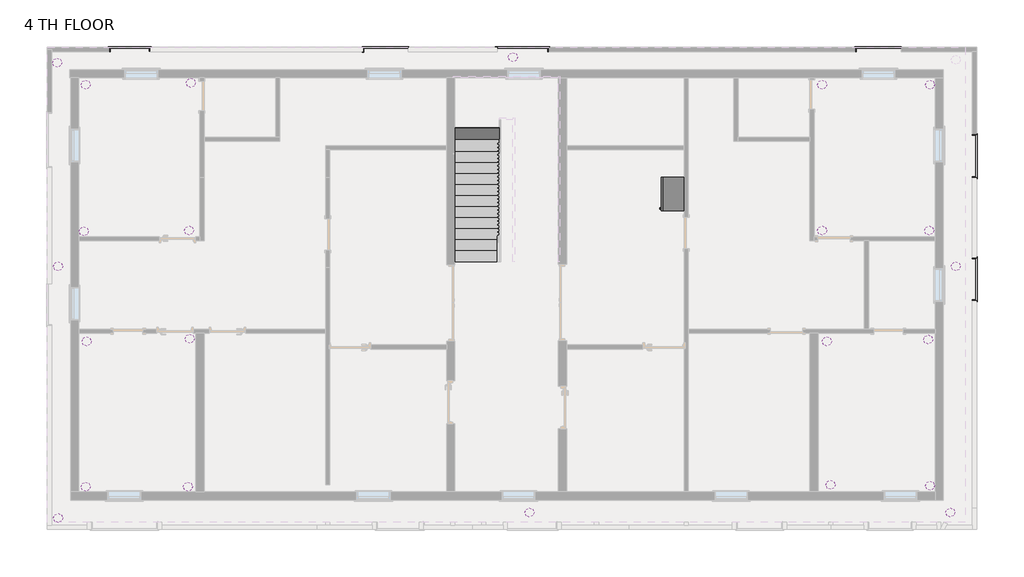
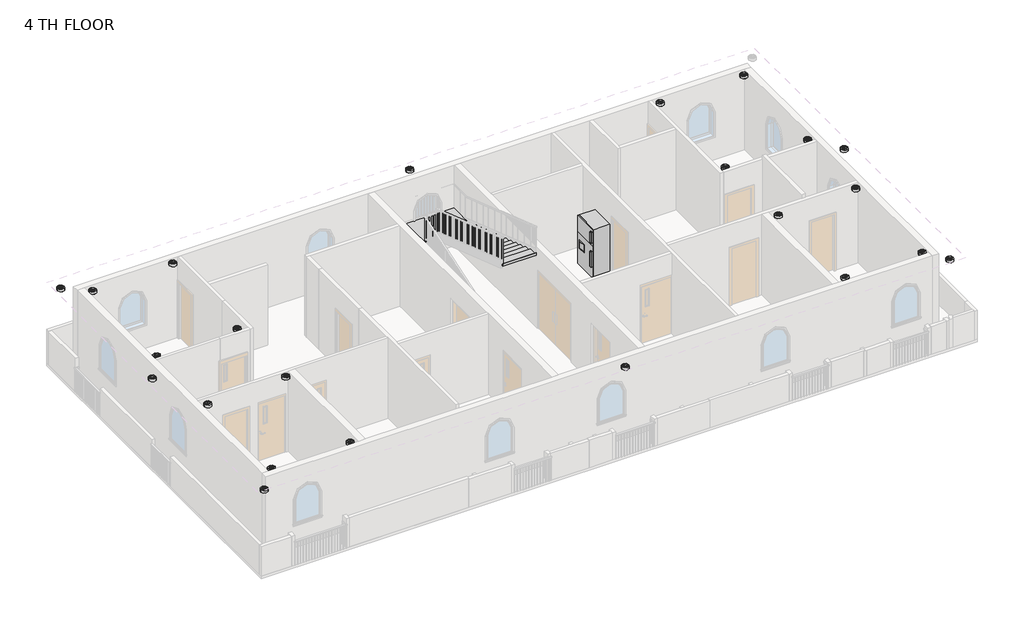
# One storey, part 6 of 7: 23 light fixtures, 6 railings, 1 furniture element, 1 stair flight.
"""IFC4 building model written with IfcOpenShell, lengths in millimetres."""

from ifc_helpers import new_model, si_unit, frame, origin, place, context, project, spatial, polyline, outline, extrude, faceted_brep, transform, mapped, element, save
from components import furniture_65fa61b5, ceiling_light_flat_round_60w_120v_7c4c2a52, stair_flight_ccf7fef2

model = new_model("IFC4")

# Units and contexts
model_context = context("Model", 3, world=origin())
ifc_project = project(units=[si_unit("LENGTHUNIT", "METRE", prefix="MILLI")], contexts=[model_context])

# Site, building, storey
site = spatial("IfcSite", under=ifc_project)
building = spatial("IfcBuilding", under=site)
storey = spatial("IfcBuildingStorey", under=building, Name="4 TH FLOOR", Elevation=12801.6)

# Furniture
placement = place(None, origin())
furniture_shape = furniture_65fa61b5(model_context)
element("IfcFurniture", 1, at=placement, inside=storey, context=model_context, shape_type="MappedRepresentation", body=[
    mapped(furniture_shape, transform((4507.551208, 3815.4567334, 12801.6), x_axis=(0.0, -1.0, 0.0), y_axis=(1.0, 0.0, 0.0), z_axis=(0.0, 0.0, 1.0))),
])

# Light fixtures
ceiling_light_flat_round_60w_120v_shape = ceiling_light_flat_round_60w_120v_7c4c2a52(model_context)
element("IfcLightFixture", 2, ObjectType="Ceiling Light - Flat Round : 60W - 120V", at=placement, inside=storey, context=model_context, shape_type="MappedRepresentation", body=[
    mapped(ceiling_light_flat_round_60w_120v_shape, transform((-12821.5987925, 8050.9067329, 13411.2), x_axis=(1.0, 0.0, 0.0), y_axis=(0.0, 1.0, 0.0), z_axis=(0.0, 0.0, 1.0))),
])
element("IfcLightFixture", 3, ObjectType="Ceiling Light - Flat Round : 60W - 120V", at=placement, inside=storey, context=model_context, shape_type="MappedRepresentation", body=[
    mapped(ceiling_light_flat_round_60w_120v_shape, transform((-249.1067989, 8203.3067329, 13411.2), x_axis=(1.0, 0.0, 0.0), y_axis=(0.0, 1.0, 0.0), z_axis=(0.0, 0.0, 1.0))),
])
element("IfcLightFixture", 4, ObjectType="Ceiling Light - Flat Round : 60W - 120V", at=placement, inside=storey, context=model_context, shape_type="MappedRepresentation", body=[
    mapped(ceiling_light_flat_round_60w_120v_shape, transform((-12796.1987925, -4509.3932193, 13411.2), x_axis=(1.0, 0.0, 0.0), y_axis=(0.0, 1.0, 0.0), z_axis=(0.0, 0.0, 1.0))),
])
element("IfcLightFixture", 5, ObjectType="Ceiling Light - Flat Round : 60W - 120V", at=placement, inside=storey, context=model_context, shape_type="MappedRepresentation", body=[
    mapped(ceiling_light_flat_round_60w_120v_shape, transform((-12796.1987925, 2431.1567332, 13411.2), x_axis=(1.0, 0.0, 0.0), y_axis=(0.0, 1.0, 0.0), z_axis=(0.0, 0.0, 1.0))),
])
element("IfcLightFixture", 6, ObjectType="Ceiling Light - Flat Round : 60W - 120V", at=placement, inside=storey, context=model_context, shape_type="MappedRepresentation", body=[
    mapped(ceiling_light_flat_round_60w_120v_shape, transform((208.0932011, -4356.9932193, 13411.2), x_axis=(1.0, 0.0, 0.0), y_axis=(0.0, 1.0, 0.0), z_axis=(0.0, 0.0, 1.0))),
])
element("IfcLightFixture", 7, ObjectType="Ceiling Light - Flat Round : 60W - 120V", at=placement, inside=storey, context=model_context, shape_type="MappedRepresentation", body=[
    mapped(ceiling_light_flat_round_60w_120v_shape, transform((11816.4012075, -4356.9932193, 13411.2), x_axis=(1.0, 0.0, 0.0), y_axis=(0.0, 1.0, 0.0), z_axis=(0.0, 0.0, 1.0))),
])
element("IfcLightFixture", 8, ObjectType="Ceiling Light - Flat Round : 60W - 120V", at=placement, inside=storey, context=model_context, shape_type="MappedRepresentation", body=[
    mapped(ceiling_light_flat_round_60w_120v_shape, transform((11968.8012075, 2431.1567332, 13411.2), x_axis=(1.0, 0.0, 0.0), y_axis=(0.0, 1.0, 0.0), z_axis=(0.0, 0.0, 1.0))),
])
element("IfcLightFixture", 9, ObjectType="Ceiling Light - Flat Round : 60W - 120V", at=placement, inside=storey, context=model_context, shape_type="MappedRepresentation", body=[
    mapped(ceiling_light_flat_round_60w_120v_shape, transform((8279.4512079, 7441.3067329, 13411.2), x_axis=(1.0, 0.0, 0.0), y_axis=(0.0, 1.0, 0.0), z_axis=(0.0, 0.0, 1.0))),
])
element("IfcLightFixture", 10, ObjectType="Ceiling Light - Flat Round : 60W - 120V", at=placement, inside=storey, context=model_context, shape_type="MappedRepresentation", body=[
    mapped(ceiling_light_flat_round_60w_120v_shape, transform((11257.6012075, 7441.3067329, 13411.2), x_axis=(1.0, 0.0, 0.0), y_axis=(0.0, 1.0, 0.0), z_axis=(0.0, 0.0, 1.0))),
])
element("IfcLightFixture", 11, ObjectType="Ceiling Light - Flat Round : 60W - 120V", at=placement, inside=storey, context=model_context, shape_type="MappedRepresentation", body=[
    mapped(ceiling_light_flat_round_60w_120v_shape, transform((8279.4512079, 3421.7567332, 13411.2), x_axis=(1.0, 0.0, 0.0), y_axis=(0.0, 1.0, 0.0), z_axis=(0.0, 0.0, 1.0))),
])
element("IfcLightFixture", 12, ObjectType="Ceiling Light - Flat Round : 60W - 120V", at=placement, inside=storey, context=model_context, shape_type="MappedRepresentation", body=[
    mapped(ceiling_light_flat_round_60w_120v_shape, transform((11232.2012075, 3421.7567332, 13411.2), x_axis=(1.0, 0.0, 0.0), y_axis=(0.0, 1.0, 0.0), z_axis=(0.0, 0.0, 1.0))),
])
element("IfcLightFixture", 13, ObjectType="Ceiling Light - Flat Round : 60W - 120V", at=placement, inside=storey, context=model_context, shape_type="MappedRepresentation", body=[
    mapped(ceiling_light_flat_round_60w_120v_shape, transform((8412.8012079, 361.0567334, 13411.2), x_axis=(1.0, 0.0, 0.0), y_axis=(0.0, 1.0, 0.0), z_axis=(0.0, 0.0, 1.0))),
])
element("IfcLightFixture", 14, ObjectType="Ceiling Light - Flat Round : 60W - 120V", at=placement, inside=storey, context=model_context, shape_type="MappedRepresentation", body=[
    mapped(ceiling_light_flat_round_60w_120v_shape, transform((11206.8012075, 411.8567334, 13411.2), x_axis=(1.0, 0.0, 0.0), y_axis=(0.0, 1.0, 0.0), z_axis=(0.0, 0.0, 1.0))),
])
element("IfcLightFixture", 15, ObjectType="Ceiling Light - Flat Round : 60W - 120V", at=placement, inside=storey, context=model_context, shape_type="MappedRepresentation", body=[
    mapped(ceiling_light_flat_round_60w_120v_shape, transform((8514.4012079, -3594.9932193, 13411.2), x_axis=(1.0, 0.0, 0.0), y_axis=(0.0, 1.0, 0.0), z_axis=(0.0, 0.0, 1.0))),
])
element("IfcLightFixture", 16, ObjectType="Ceiling Light - Flat Round : 60W - 120V", at=placement, inside=storey, context=model_context, shape_type="MappedRepresentation", body=[
    mapped(ceiling_light_flat_round_60w_120v_shape, transform((11257.6012075, -3620.3932193, 13411.2), x_axis=(1.0, 0.0, 0.0), y_axis=(0.0, 1.0, 0.0), z_axis=(0.0, 0.0, 1.0))),
])
element("IfcLightFixture", 17, ObjectType="Ceiling Light - Flat Round : 60W - 120V", at=placement, inside=storey, context=model_context, shape_type="MappedRepresentation", body=[
    mapped(ceiling_light_flat_round_60w_120v_shape, transform((-12008.7987925, 361.0567334, 13411.2), x_axis=(1.0, 0.0, 0.0), y_axis=(0.0, 1.0, 0.0), z_axis=(0.0, 0.0, 1.0))),
])
element("IfcLightFixture", 18, ObjectType="Ceiling Light - Flat Round : 60W - 120V", at=placement, inside=storey, context=model_context, shape_type="MappedRepresentation", body=[
    mapped(ceiling_light_flat_round_60w_120v_shape, transform((-9163.9987992, 437.2567334, 13411.2), x_axis=(1.0, 0.0, 0.0), y_axis=(0.0, 1.0, 0.0), z_axis=(0.0, 0.0, 1.0))),
])
element("IfcLightFixture", 19, ObjectType="Ceiling Light - Flat Round : 60W - 120V", at=placement, inside=storey, context=model_context, shape_type="MappedRepresentation", body=[
    mapped(ceiling_light_flat_round_60w_120v_shape, transform((-12034.1987925, -3645.7932193, 13411.2), x_axis=(1.0, 0.0, 0.0), y_axis=(0.0, 1.0, 0.0), z_axis=(0.0, 0.0, 1.0))),
])
element("IfcLightFixture", 20, ObjectType="Ceiling Light - Flat Round : 60W - 120V", at=placement, inside=storey, context=model_context, shape_type="MappedRepresentation", body=[
    mapped(ceiling_light_flat_round_60w_120v_shape, transform((-9214.7987992, -3645.7932193, 13411.2), x_axis=(1.0, 0.0, 0.0), y_axis=(0.0, 1.0, 0.0), z_axis=(0.0, 0.0, 1.0))),
])
element("IfcLightFixture", 21, ObjectType="Ceiling Light - Flat Round : 60W - 120V", at=placement, inside=storey, context=model_context, shape_type="MappedRepresentation", body=[
    mapped(ceiling_light_flat_round_60w_120v_shape, transform((-12034.1987925, 7441.3067329, 13411.2), x_axis=(1.0, 0.0, 0.0), y_axis=(0.0, 1.0, 0.0), z_axis=(0.0, 0.0, 1.0))),
])
element("IfcLightFixture", 22, ObjectType="Ceiling Light - Flat Round : 60W - 120V", at=placement, inside=storey, context=model_context, shape_type="MappedRepresentation", body=[
    mapped(ceiling_light_flat_round_60w_120v_shape, transform((-9132.2487992, 7492.1067329, 13411.2), x_axis=(1.0, 0.0, 0.0), y_axis=(0.0, 1.0, 0.0), z_axis=(0.0, 0.0, 1.0))),
])
element("IfcLightFixture", 23, ObjectType="Ceiling Light - Flat Round : 60W - 120V", at=placement, inside=storey, context=model_context, shape_type="MappedRepresentation", body=[
    mapped(ceiling_light_flat_round_60w_120v_shape, transform((-12084.9987925, 3396.3567332, 13411.2), x_axis=(1.0, 0.0, 0.0), y_axis=(0.0, 1.0, 0.0), z_axis=(0.0, 0.0, 1.0))),
])
element("IfcLightFixture", 24, ObjectType="Ceiling Light - Flat Round : 60W - 120V", at=placement, inside=storey, context=model_context, shape_type="MappedRepresentation", body=[
    mapped(ceiling_light_flat_round_60w_120v_shape, transform((-9183.0487992, 3421.7567332, 13411.2), x_axis=(1.0, 0.0, 0.0), y_axis=(0.0, 1.0, 0.0), z_axis=(0.0, 0.0, 1.0))),
])

# Railings
element("IfcRailing", 25, ObjectType="Handrail - Rectangular", at=placement, inside=storey, context=model_context, shape_type="SolidModel", body=[
    faceted_brep([(-11412.4067989, 8355.7067329, 13716.0), (-11412.4067989, 8355.7067329, 13665.2), (-11361.6067989, 8355.7067329, 13665.2), (-11361.6067989, 8355.7067329, 13716.0), (-11412.4067989, 8495.4067329, 13716.0), (-11412.4067989, 8495.4067329, 13665.2), (-11361.6067989, 8444.6067329, 13665.2), (-11361.6067989, 8444.6067329, 13716.0), (-10231.3067989, 8495.4067329, 13716.0), (-10231.3067989, 8495.4067329, 13665.2), (-10282.1067989, 8444.6067329, 13665.2), (-10282.1067989, 8444.6067329, 13716.0), (-10231.3067989, 8368.4067329, 13716.0), (-10282.1067989, 8368.4067329, 13716.0), (-10282.1067989, 8368.4067329, 13665.2), (-10231.3067989, 8368.4067329, 13665.2)], [[[0, 1, 2, 3]], [[1, 0, 4, 5]], [[2, 1, 5, 6]], [[3, 2, 6, 7]], [[0, 3, 7, 4]], [[5, 4, 8, 9]], [[6, 5, 9, 10]], [[7, 6, 10, 11]], [[4, 7, 11, 8]], [[12, 13, 14, 15]], [[9, 8, 12, 15]], [[10, 9, 15, 14]], [[11, 10, 14, 13]], [[8, 11, 13, 12]]]),
    extrude(outline(polyline([(-10278.9317989, 8460.4817329), (-10278.9317989, 8479.5317329), (-10259.8817989, 8479.5317329), (-10259.8817989, 8460.4817329), (-10278.9317989, 8460.4817329)])), frame((0.0, 0.0, 12801.6), z_axis=(0.0, 0.0, 1.0), x_axis=(1.0, 0.0, 0.0)), (0.0, 0.0, 1.0), 863.6),
    extrude(outline(polyline([(-10380.5317989, 8460.4817329), (-10380.5317989, 8479.5317329), (-10361.4817989, 8479.5317329), (-10361.4817989, 8460.4817329), (-10380.5317989, 8460.4817329)])), frame((0.0, 0.0, 12801.6), z_axis=(0.0, 0.0, 1.0), x_axis=(1.0, 0.0, 0.0)), (0.0, 0.0, 1.0), 863.6),
    extrude(outline(polyline([(-10482.1317989, 8460.4817329), (-10482.1317989, 8479.5317329), (-10463.0817989, 8479.5317329), (-10463.0817989, 8460.4817329), (-10482.1317989, 8460.4817329)])), frame((0.0, 0.0, 12801.6), z_axis=(0.0, 0.0, 1.0), x_axis=(1.0, 0.0, 0.0)), (0.0, 0.0, 1.0), 863.6),
    extrude(outline(polyline([(-10583.7317989, 8460.4817329), (-10583.7317989, 8479.5317329), (-10564.6817989, 8479.5317329), (-10564.6817989, 8460.4817329), (-10583.7317989, 8460.4817329)])), frame((0.0, 0.0, 12801.6), z_axis=(0.0, 0.0, 1.0), x_axis=(1.0, 0.0, 0.0)), (0.0, 0.0, 1.0), 863.6),
    extrude(outline(polyline([(-10685.3317989, 8460.4817329), (-10685.3317989, 8479.5317329), (-10666.2817989, 8479.5317329), (-10666.2817989, 8460.4817329), (-10685.3317989, 8460.4817329)])), frame((0.0, 0.0, 12801.6), z_axis=(0.0, 0.0, 1.0), x_axis=(1.0, 0.0, 0.0)), (0.0, 0.0, 1.0), 863.6),
    extrude(outline(polyline([(-10786.9317989, 8460.4817329), (-10786.9317989, 8479.5317329), (-10767.8817989, 8479.5317329), (-10767.8817989, 8460.4817329), (-10786.9317989, 8460.4817329)])), frame((0.0, 0.0, 12801.6), z_axis=(0.0, 0.0, 1.0), x_axis=(1.0, 0.0, 0.0)), (0.0, 0.0, 1.0), 863.6),
    extrude(outline(polyline([(-10888.5317989, 8460.4817329), (-10888.5317989, 8479.5317329), (-10869.4817989, 8479.5317329), (-10869.4817989, 8460.4817329), (-10888.5317989, 8460.4817329)])), frame((0.0, 0.0, 12801.6), z_axis=(0.0, 0.0, 1.0), x_axis=(1.0, 0.0, 0.0)), (0.0, 0.0, 1.0), 863.6),
    extrude(outline(polyline([(-10990.1317989, 8460.4817329), (-10990.1317989, 8479.5317329), (-10971.0817989, 8479.5317329), (-10971.0817989, 8460.4817329), (-10990.1317989, 8460.4817329)])), frame((0.0, 0.0, 12801.6), z_axis=(0.0, 0.0, 1.0), x_axis=(1.0, 0.0, 0.0)), (0.0, 0.0, 1.0), 863.6),
    extrude(outline(polyline([(-11091.7317989, 8460.4817329), (-11091.7317989, 8479.5317329), (-11072.6817989, 8479.5317329), (-11072.6817989, 8460.4817329), (-11091.7317989, 8460.4817329)])), frame((0.0, 0.0, 12801.6), z_axis=(0.0, 0.0, 1.0), x_axis=(1.0, 0.0, 0.0)), (0.0, 0.0, 1.0), 863.6),
    extrude(outline(polyline([(-11193.3317989, 8460.4817329), (-11193.3317989, 8479.5317329), (-11174.2817989, 8479.5317329), (-11174.2817989, 8460.4817329), (-11193.3317989, 8460.4817329)])), frame((0.0, 0.0, 12801.6), z_axis=(0.0, 0.0, 1.0), x_axis=(1.0, 0.0, 0.0)), (0.0, 0.0, 1.0), 863.6),
    extrude(outline(polyline([(-11294.9317989, 8460.4817329), (-11294.9317989, 8479.5317329), (-11275.8817989, 8479.5317329), (-11275.8817989, 8460.4817329), (-11294.9317989, 8460.4817329)])), frame((0.0, 0.0, 12801.6), z_axis=(0.0, 0.0, 1.0), x_axis=(1.0, 0.0, 0.0)), (0.0, 0.0, 1.0), 863.6),
    extrude(outline(polyline([(-11377.4817989, 8447.7817329), (-11396.5317989, 8447.7817329), (-11396.5317989, 8466.8317329), (-11377.4817989, 8466.8317329), (-11377.4817989, 8447.7817329)])), frame((0.0, 0.0, 12801.6), z_axis=(0.0, 0.0, 1.0), x_axis=(1.0, 0.0, 0.0)), (0.0, 0.0, 1.0), 863.6),
    extrude(outline(polyline([(-10266.2317989, 8460.4817329), (-10266.2317989, 8479.5317329), (-10247.1817989, 8479.5317329), (-10247.1817989, 8460.4817329), (-10266.2317989, 8460.4817329)])), frame((0.0, 0.0, 12801.6), z_axis=(0.0, 0.0, 1.0), x_axis=(1.0, 0.0, 0.0)), (0.0, 0.0, 1.0), 863.6),
    extrude(outline(polyline([(-11377.4817989, 8460.4817329), (-11396.5317989, 8460.4817329), (-11396.5317989, 8479.5317329), (-11377.4817989, 8479.5317329), (-11377.4817989, 8460.4817329)])), frame((0.0, 0.0, 12801.6), z_axis=(0.0, 0.0, 1.0), x_axis=(1.0, 0.0, 0.0)), (0.0, 0.0, 1.0), 863.6),
    extrude(outline(polyline([(-10266.2317989, 8387.4567329), (-10247.1817989, 8387.4567329), (-10247.1817989, 8368.4067329), (-10266.2317989, 8368.4067329), (-10266.2317989, 8387.4567329)])), frame((0.0, 0.0, 12801.6), z_axis=(0.0, 0.0, 1.0), x_axis=(1.0, 0.0, 0.0)), (0.0, 0.0, 1.0), 863.6),
    extrude(outline(polyline([(-11377.4817989, 8355.7067329), (-11396.5317989, 8355.7067329), (-11396.5317989, 8374.7567329), (-11377.4817989, 8374.7567329), (-11377.4817989, 8355.7067329)])), frame((0.0, 0.0, 12801.6), z_axis=(0.0, 0.0, 1.0), x_axis=(1.0, 0.0, 0.0)), (0.0, 0.0, 1.0), 863.6),
])
element("IfcRailing", 26, ObjectType="Handrail - Rectangular", at=placement, inside=storey, context=model_context, shape_type="SolidModel", body=[
    faceted_brep([(-4407.8487992, 8336.6567329, 13716.0), (-4407.8487992, 8336.6567329, 13665.2), (-4357.0487992, 8336.6567329, 13665.2), (-4357.0487992, 8336.6567329, 13716.0), (-4407.8487992, 8495.4067329, 13716.0), (-4407.8487992, 8495.4067329, 13665.2), (-4357.0487992, 8444.6067329, 13665.2), (-4357.0487992, 8444.6067329, 13716.0), (-3120.4490672, 8495.4067329, 13716.0), (-3120.4490672, 8444.6067329, 13716.0), (-3120.4490672, 8444.6067329, 13665.2), (-3120.4490672, 8495.4067329, 13665.2)], [[[0, 1, 2, 3]], [[1, 0, 4, 5]], [[2, 1, 5, 6]], [[3, 2, 6, 7]], [[0, 3, 7, 4]], [[8, 9, 10, 11]], [[5, 4, 8, 11]], [[6, 5, 11, 10]], [[7, 6, 10, 9]], [[4, 7, 9, 8]]]),
    extrude(outline(polyline([(-3172.7737992, 8460.4817329), (-3172.7737992, 8479.5317329), (-3153.7237992, 8479.5317329), (-3153.7237992, 8460.4817329), (-3172.7737992, 8460.4817329)])), frame((0.0, 0.0, 12801.6), z_axis=(0.0, 0.0, 1.0), x_axis=(1.0, 0.0, 0.0)), (0.0, 0.0, 1.0), 863.6),
    extrude(outline(polyline([(-3274.3737992, 8460.4817329), (-3274.3737992, 8479.5317329), (-3255.3237992, 8479.5317329), (-3255.3237992, 8460.4817329), (-3274.3737992, 8460.4817329)])), frame((0.0, 0.0, 12801.6), z_axis=(0.0, 0.0, 1.0), x_axis=(1.0, 0.0, 0.0)), (0.0, 0.0, 1.0), 863.6),
    extrude(outline(polyline([(-3375.9737992, 8460.4817329), (-3375.9737992, 8479.5317329), (-3356.9237992, 8479.5317329), (-3356.9237992, 8460.4817329), (-3375.9737992, 8460.4817329)])), frame((0.0, 0.0, 12801.6), z_axis=(0.0, 0.0, 1.0), x_axis=(1.0, 0.0, 0.0)), (0.0, 0.0, 1.0), 863.6),
    extrude(outline(polyline([(-3477.5737992, 8460.4817329), (-3477.5737992, 8479.5317329), (-3458.5237992, 8479.5317329), (-3458.5237992, 8460.4817329), (-3477.5737992, 8460.4817329)])), frame((0.0, 0.0, 12801.6), z_axis=(0.0, 0.0, 1.0), x_axis=(1.0, 0.0, 0.0)), (0.0, 0.0, 1.0), 863.6),
    extrude(outline(polyline([(-3579.1737992, 8460.4817329), (-3579.1737992, 8479.5317329), (-3560.1237992, 8479.5317329), (-3560.1237992, 8460.4817329), (-3579.1737992, 8460.4817329)])), frame((0.0, 0.0, 12801.6), z_axis=(0.0, 0.0, 1.0), x_axis=(1.0, 0.0, 0.0)), (0.0, 0.0, 1.0), 863.6),
    extrude(outline(polyline([(-3680.7737992, 8460.4817329), (-3680.7737992, 8479.5317329), (-3661.7237992, 8479.5317329), (-3661.7237992, 8460.4817329), (-3680.7737992, 8460.4817329)])), frame((0.0, 0.0, 12801.6), z_axis=(0.0, 0.0, 1.0), x_axis=(1.0, 0.0, 0.0)), (0.0, 0.0, 1.0), 863.6),
    extrude(outline(polyline([(-3782.3737992, 8460.4817329), (-3782.3737992, 8479.5317329), (-3763.3237992, 8479.5317329), (-3763.3237992, 8460.4817329), (-3782.3737992, 8460.4817329)])), frame((0.0, 0.0, 12801.6), z_axis=(0.0, 0.0, 1.0), x_axis=(1.0, 0.0, 0.0)), (0.0, 0.0, 1.0), 863.6),
    extrude(outline(polyline([(-3883.9737992, 8460.4817329), (-3883.9737992, 8479.5317329), (-3864.9237992, 8479.5317329), (-3864.9237992, 8460.4817329), (-3883.9737992, 8460.4817329)])), frame((0.0, 0.0, 12801.6), z_axis=(0.0, 0.0, 1.0), x_axis=(1.0, 0.0, 0.0)), (0.0, 0.0, 1.0), 863.6),
    extrude(outline(polyline([(-3985.5737992, 8460.4817329), (-3985.5737992, 8479.5317329), (-3966.5237992, 8479.5317329), (-3966.5237992, 8460.4817329), (-3985.5737992, 8460.4817329)])), frame((0.0, 0.0, 12801.6), z_axis=(0.0, 0.0, 1.0), x_axis=(1.0, 0.0, 0.0)), (0.0, 0.0, 1.0), 863.6),
    extrude(outline(polyline([(-4087.1737992, 8460.4817329), (-4087.1737992, 8479.5317329), (-4068.1237992, 8479.5317329), (-4068.1237992, 8460.4817329), (-4087.1737992, 8460.4817329)])), frame((0.0, 0.0, 12801.6), z_axis=(0.0, 0.0, 1.0), x_axis=(1.0, 0.0, 0.0)), (0.0, 0.0, 1.0), 863.6),
    extrude(outline(polyline([(-4188.7737992, 8460.4817329), (-4188.7737992, 8479.5317329), (-4169.7237992, 8479.5317329), (-4169.7237992, 8460.4817329), (-4188.7737992, 8460.4817329)])), frame((0.0, 0.0, 12801.6), z_axis=(0.0, 0.0, 1.0), x_axis=(1.0, 0.0, 0.0)), (0.0, 0.0, 1.0), 863.6),
    extrude(outline(polyline([(-4290.3737992, 8460.4817329), (-4290.3737992, 8479.5317329), (-4271.3237992, 8479.5317329), (-4271.3237992, 8460.4817329), (-4290.3737992, 8460.4817329)])), frame((0.0, 0.0, 12801.6), z_axis=(0.0, 0.0, 1.0), x_axis=(1.0, 0.0, 0.0)), (0.0, 0.0, 1.0), 863.6),
    extrude(outline(polyline([(-4372.9237992, 8428.7317329), (-4391.9737992, 8428.7317329), (-4391.9737992, 8447.7817329), (-4372.9237992, 8447.7817329), (-4372.9237992, 8428.7317329)])), frame((0.0, 0.0, 12801.6), z_axis=(0.0, 0.0, 1.0), x_axis=(1.0, 0.0, 0.0)), (0.0, 0.0, 1.0), 863.6),
    extrude(outline(polyline([(-4372.9237992, 8460.4817329), (-4391.9737992, 8460.4817329), (-4391.9737992, 8479.5317329), (-4372.9237992, 8479.5317329), (-4372.9237992, 8460.4817329)])), frame((0.0, 0.0, 12801.6), z_axis=(0.0, 0.0, 1.0), x_axis=(1.0, 0.0, 0.0)), (0.0, 0.0, 1.0), 863.6),
    extrude(outline(polyline([(-3139.4990672, 8460.4817329), (-3139.4990672, 8479.5317329), (-3120.4490672, 8479.5317329), (-3120.4490672, 8460.4817329), (-3139.4990672, 8460.4817329)])), frame((0.0, 0.0, 12801.6), z_axis=(0.0, 0.0, 1.0), x_axis=(1.0, 0.0, 0.0)), (0.0, 0.0, 1.0), 863.6),
    extrude(outline(polyline([(-4372.9237992, 8336.6567329), (-4391.9737992, 8336.6567329), (-4391.9737992, 8355.7067329), (-4372.9237992, 8355.7067329), (-4372.9237992, 8336.6567329)])), frame((0.0, 0.0, 12801.6), z_axis=(0.0, 0.0, 1.0), x_axis=(1.0, 0.0, 0.0)), (0.0, 0.0, 1.0), 863.6),
])
element("IfcRailing", 27, ObjectType="Handrail - Rectangular", at=placement, inside=storey, context=model_context, shape_type="SolidModel", body=[
    faceted_brep([(-732.8490672, 8355.7067329, 13716.0), (-732.8490672, 8355.7067329, 13665.2), (-682.0490672, 8355.7067329, 13665.2), (-682.0490672, 8355.7067329, 13716.0), (-732.8490672, 8495.4067329, 13716.0), (-732.8490672, 8495.4067329, 13665.2), (-682.0490672, 8444.6067329, 13665.2), (-682.0490672, 8444.6067329, 13716.0), (766.8932011, 8495.4067329, 13716.0), (766.8932011, 8495.4067329, 13665.2), (716.0932011, 8444.6067329, 13665.2), (716.0932011, 8444.6067329, 13716.0), (766.8932011, 8355.7067329, 13716.0), (716.0932011, 8355.7067329, 13716.0), (716.0932011, 8355.7067329, 13665.2), (766.8932011, 8355.7067329, 13665.2)], [[[0, 1, 2, 3]], [[1, 0, 4, 5]], [[2, 1, 5, 6]], [[3, 2, 6, 7]], [[0, 3, 7, 4]], [[5, 4, 8, 9]], [[6, 5, 9, 10]], [[7, 6, 10, 11]], [[4, 7, 11, 8]], [[12, 13, 14, 15]], [[9, 8, 12, 15]], [[10, 9, 15, 14]], [[11, 10, 14, 13]], [[8, 11, 13, 12]]]),
    extrude(outline(polyline([(731.9682011, 8377.9317329), (751.0182011, 8377.9317329), (751.0182011, 8358.8817329), (731.9682011, 8358.8817329), (731.9682011, 8377.9317329)])), frame((0.0, 0.0, 12801.6), z_axis=(0.0, 0.0, 1.0), x_axis=(1.0, 0.0, 0.0)), (0.0, 0.0, 1.0), 863.6),
    extrude(outline(polyline([(705.4259328, 8460.4817329), (705.4259328, 8479.5317329), (724.4759328, 8479.5317329), (724.4759328, 8460.4817329), (705.4259328, 8460.4817329)])), frame((0.0, 0.0, 12801.6), z_axis=(0.0, 0.0, 1.0), x_axis=(1.0, 0.0, 0.0)), (0.0, 0.0, 1.0), 863.6),
    extrude(outline(polyline([(603.8259328, 8460.4817329), (603.8259328, 8479.5317329), (622.8759328, 8479.5317329), (622.8759328, 8460.4817329), (603.8259328, 8460.4817329)])), frame((0.0, 0.0, 12801.6), z_axis=(0.0, 0.0, 1.0), x_axis=(1.0, 0.0, 0.0)), (0.0, 0.0, 1.0), 863.6),
    extrude(outline(polyline([(502.2259328, 8460.4817329), (502.2259328, 8479.5317329), (521.2759328, 8479.5317329), (521.2759328, 8460.4817329), (502.2259328, 8460.4817329)])), frame((0.0, 0.0, 12801.6), z_axis=(0.0, 0.0, 1.0), x_axis=(1.0, 0.0, 0.0)), (0.0, 0.0, 1.0), 863.6),
    extrude(outline(polyline([(400.6259328, 8460.4817329), (400.6259328, 8479.5317329), (419.6759328, 8479.5317329), (419.6759328, 8460.4817329), (400.6259328, 8460.4817329)])), frame((0.0, 0.0, 12801.6), z_axis=(0.0, 0.0, 1.0), x_axis=(1.0, 0.0, 0.0)), (0.0, 0.0, 1.0), 863.6),
    extrude(outline(polyline([(299.0259328, 8460.4817329), (299.0259328, 8479.5317329), (318.0759328, 8479.5317329), (318.0759328, 8460.4817329), (299.0259328, 8460.4817329)])), frame((0.0, 0.0, 12801.6), z_axis=(0.0, 0.0, 1.0), x_axis=(1.0, 0.0, 0.0)), (0.0, 0.0, 1.0), 863.6),
    extrude(outline(polyline([(197.4259328, 8460.4817329), (197.4259328, 8479.5317329), (216.4759328, 8479.5317329), (216.4759328, 8460.4817329), (197.4259328, 8460.4817329)])), frame((0.0, 0.0, 12801.6), z_axis=(0.0, 0.0, 1.0), x_axis=(1.0, 0.0, 0.0)), (0.0, 0.0, 1.0), 863.6),
    extrude(outline(polyline([(95.8259328, 8460.4817329), (95.8259328, 8479.5317329), (114.8759328, 8479.5317329), (114.8759328, 8460.4817329), (95.8259328, 8460.4817329)])), frame((0.0, 0.0, 12801.6), z_axis=(0.0, 0.0, 1.0), x_axis=(1.0, 0.0, 0.0)), (0.0, 0.0, 1.0), 863.6),
    extrude(outline(polyline([(-5.7740672, 8460.4817329), (-5.7740672, 8479.5317329), (13.2759328, 8479.5317329), (13.2759328, 8460.4817329), (-5.7740672, 8460.4817329)])), frame((0.0, 0.0, 12801.6), z_axis=(0.0, 0.0, 1.0), x_axis=(1.0, 0.0, 0.0)), (0.0, 0.0, 1.0), 863.6),
    extrude(outline(polyline([(-107.3740672, 8460.4817329), (-107.3740672, 8479.5317329), (-88.3240672, 8479.5317329), (-88.3240672, 8460.4817329), (-107.3740672, 8460.4817329)])), frame((0.0, 0.0, 12801.6), z_axis=(0.0, 0.0, 1.0), x_axis=(1.0, 0.0, 0.0)), (0.0, 0.0, 1.0), 863.6),
    extrude(outline(polyline([(-208.9740672, 8460.4817329), (-208.9740672, 8479.5317329), (-189.9240672, 8479.5317329), (-189.9240672, 8460.4817329), (-208.9740672, 8460.4817329)])), frame((0.0, 0.0, 12801.6), z_axis=(0.0, 0.0, 1.0), x_axis=(1.0, 0.0, 0.0)), (0.0, 0.0, 1.0), 863.6),
    extrude(outline(polyline([(-310.5740672, 8460.4817329), (-310.5740672, 8479.5317329), (-291.5240672, 8479.5317329), (-291.5240672, 8460.4817329), (-310.5740672, 8460.4817329)])), frame((0.0, 0.0, 12801.6), z_axis=(0.0, 0.0, 1.0), x_axis=(1.0, 0.0, 0.0)), (0.0, 0.0, 1.0), 863.6),
    extrude(outline(polyline([(-412.1740672, 8460.4817329), (-412.1740672, 8479.5317329), (-393.1240672, 8479.5317329), (-393.1240672, 8460.4817329), (-412.1740672, 8460.4817329)])), frame((0.0, 0.0, 12801.6), z_axis=(0.0, 0.0, 1.0), x_axis=(1.0, 0.0, 0.0)), (0.0, 0.0, 1.0), 863.6),
    extrude(outline(polyline([(-513.7740672, 8460.4817329), (-513.7740672, 8479.5317329), (-494.7240672, 8479.5317329), (-494.7240672, 8460.4817329), (-513.7740672, 8460.4817329)])), frame((0.0, 0.0, 12801.6), z_axis=(0.0, 0.0, 1.0), x_axis=(1.0, 0.0, 0.0)), (0.0, 0.0, 1.0), 863.6),
    extrude(outline(polyline([(-615.3740672, 8460.4817329), (-615.3740672, 8479.5317329), (-596.3240672, 8479.5317329), (-596.3240672, 8460.4817329), (-615.3740672, 8460.4817329)])), frame((0.0, 0.0, 12801.6), z_axis=(0.0, 0.0, 1.0), x_axis=(1.0, 0.0, 0.0)), (0.0, 0.0, 1.0), 863.6),
    extrude(outline(polyline([(-697.9240672, 8447.7817329), (-716.9740672, 8447.7817329), (-716.9740672, 8466.8317329), (-697.9240672, 8466.8317329), (-697.9240672, 8447.7817329)])), frame((0.0, 0.0, 12801.6), z_axis=(0.0, 0.0, 1.0), x_axis=(1.0, 0.0, 0.0)), (0.0, 0.0, 1.0), 863.6),
    extrude(outline(polyline([(731.9682011, 8460.4817329), (731.9682011, 8479.5317329), (751.0182011, 8479.5317329), (751.0182011, 8460.4817329), (731.9682011, 8460.4817329)])), frame((0.0, 0.0, 12801.6), z_axis=(0.0, 0.0, 1.0), x_axis=(1.0, 0.0, 0.0)), (0.0, 0.0, 1.0), 863.6),
    extrude(outline(polyline([(-697.9240672, 8460.4817329), (-716.9740672, 8460.4817329), (-716.9740672, 8479.5317329), (-697.9240672, 8479.5317329), (-697.9240672, 8460.4817329)])), frame((0.0, 0.0, 12801.6), z_axis=(0.0, 0.0, 1.0), x_axis=(1.0, 0.0, 0.0)), (0.0, 0.0, 1.0), 863.6),
    extrude(outline(polyline([(731.9682011, 8374.7567329), (751.0182011, 8374.7567329), (751.0182011, 8355.7067329), (731.9682011, 8355.7067329), (731.9682011, 8374.7567329)])), frame((0.0, 0.0, 12801.6), z_axis=(0.0, 0.0, 1.0), x_axis=(1.0, 0.0, 0.0)), (0.0, 0.0, 1.0), 863.6),
    extrude(outline(polyline([(-697.9240672, 8355.7067329), (-716.9740672, 8355.7067329), (-716.9740672, 8374.7567329), (-697.9240672, 8374.7567329), (-697.9240672, 8355.7067329)])), frame((0.0, 0.0, 12801.6), z_axis=(0.0, 0.0, 1.0), x_axis=(1.0, 0.0, 0.0)), (0.0, 0.0, 1.0), 863.6),
])
element("IfcRailing", 28, ObjectType="Handrail - Rectangular", at=placement, inside=storey, context=model_context, shape_type="SolidModel", body=[
    faceted_brep([(9174.2932011, 8355.7067329, 13716.0), (9174.2932011, 8355.7067329, 13665.2), (9225.0932011, 8355.7067329, 13665.2), (9225.0932011, 8355.7067329, 13716.0), (9174.2932011, 8495.4067329, 13716.0), (9174.2932011, 8495.4067329, 13665.2), (9225.0932011, 8444.6067329, 13665.2), (9225.0932011, 8444.6067329, 13716.0), (10462.2009401, 8495.4067329, 13716.0), (10462.2009401, 8444.6067329, 13716.0), (10462.2009401, 8444.6067329, 13665.2), (10462.2009401, 8495.4067329, 13665.2)], [[[0, 1, 2, 3]], [[1, 0, 4, 5]], [[2, 1, 5, 6]], [[3, 2, 6, 7]], [[0, 3, 7, 4]], [[8, 9, 10, 11]], [[5, 4, 8, 11]], [[6, 5, 11, 10]], [[7, 6, 10, 9]], [[4, 7, 9, 8]]]),
    extrude(outline(polyline([(10409.3682011, 8460.4817329), (10409.3682011, 8479.5317329), (10428.4182011, 8479.5317329), (10428.4182011, 8460.4817329), (10409.3682011, 8460.4817329)])), frame((0.0, 0.0, 12801.6), z_axis=(0.0, 0.0, 1.0), x_axis=(1.0, 0.0, 0.0)), (0.0, 0.0, 1.0), 863.6),
    extrude(outline(polyline([(10307.7682011, 8460.4817329), (10307.7682011, 8479.5317329), (10326.8182011, 8479.5317329), (10326.8182011, 8460.4817329), (10307.7682011, 8460.4817329)])), frame((0.0, 0.0, 12801.6), z_axis=(0.0, 0.0, 1.0), x_axis=(1.0, 0.0, 0.0)), (0.0, 0.0, 1.0), 863.6),
    extrude(outline(polyline([(10206.1682011, 8460.4817329), (10206.1682011, 8479.5317329), (10225.2182011, 8479.5317329), (10225.2182011, 8460.4817329), (10206.1682011, 8460.4817329)])), frame((0.0, 0.0, 12801.6), z_axis=(0.0, 0.0, 1.0), x_axis=(1.0, 0.0, 0.0)), (0.0, 0.0, 1.0), 863.6),
    extrude(outline(polyline([(10104.5682011, 8460.4817329), (10104.5682011, 8479.5317329), (10123.6182011, 8479.5317329), (10123.6182011, 8460.4817329), (10104.5682011, 8460.4817329)])), frame((0.0, 0.0, 12801.6), z_axis=(0.0, 0.0, 1.0), x_axis=(1.0, 0.0, 0.0)), (0.0, 0.0, 1.0), 863.6),
    extrude(outline(polyline([(10002.9682011, 8460.4817329), (10002.9682011, 8479.5317329), (10022.0182011, 8479.5317329), (10022.0182011, 8460.4817329), (10002.9682011, 8460.4817329)])), frame((0.0, 0.0, 12801.6), z_axis=(0.0, 0.0, 1.0), x_axis=(1.0, 0.0, 0.0)), (0.0, 0.0, 1.0), 863.6),
    extrude(outline(polyline([(9901.3682011, 8460.4817329), (9901.3682011, 8479.5317329), (9920.4182011, 8479.5317329), (9920.4182011, 8460.4817329), (9901.3682011, 8460.4817329)])), frame((0.0, 0.0, 12801.6), z_axis=(0.0, 0.0, 1.0), x_axis=(1.0, 0.0, 0.0)), (0.0, 0.0, 1.0), 863.6),
    extrude(outline(polyline([(9799.7682011, 8460.4817329), (9799.7682011, 8479.5317329), (9818.8182011, 8479.5317329), (9818.8182011, 8460.4817329), (9799.7682011, 8460.4817329)])), frame((0.0, 0.0, 12801.6), z_axis=(0.0, 0.0, 1.0), x_axis=(1.0, 0.0, 0.0)), (0.0, 0.0, 1.0), 863.6),
    extrude(outline(polyline([(9698.1682011, 8460.4817329), (9698.1682011, 8479.5317329), (9717.2182011, 8479.5317329), (9717.2182011, 8460.4817329), (9698.1682011, 8460.4817329)])), frame((0.0, 0.0, 12801.6), z_axis=(0.0, 0.0, 1.0), x_axis=(1.0, 0.0, 0.0)), (0.0, 0.0, 1.0), 863.6),
    extrude(outline(polyline([(9596.5682011, 8460.4817329), (9596.5682011, 8479.5317329), (9615.6182011, 8479.5317329), (9615.6182011, 8460.4817329), (9596.5682011, 8460.4817329)])), frame((0.0, 0.0, 12801.6), z_axis=(0.0, 0.0, 1.0), x_axis=(1.0, 0.0, 0.0)), (0.0, 0.0, 1.0), 863.6),
    extrude(outline(polyline([(9494.9682011, 8460.4817329), (9494.9682011, 8479.5317329), (9514.0182011, 8479.5317329), (9514.0182011, 8460.4817329), (9494.9682011, 8460.4817329)])), frame((0.0, 0.0, 12801.6), z_axis=(0.0, 0.0, 1.0), x_axis=(1.0, 0.0, 0.0)), (0.0, 0.0, 1.0), 863.6),
    extrude(outline(polyline([(9393.3682011, 8460.4817329), (9393.3682011, 8479.5317329), (9412.4182011, 8479.5317329), (9412.4182011, 8460.4817329), (9393.3682011, 8460.4817329)])), frame((0.0, 0.0, 12801.6), z_axis=(0.0, 0.0, 1.0), x_axis=(1.0, 0.0, 0.0)), (0.0, 0.0, 1.0), 863.6),
    extrude(outline(polyline([(9291.7682011, 8460.4817329), (9291.7682011, 8479.5317329), (9310.8182011, 8479.5317329), (9310.8182011, 8460.4817329), (9291.7682011, 8460.4817329)])), frame((0.0, 0.0, 12801.6), z_axis=(0.0, 0.0, 1.0), x_axis=(1.0, 0.0, 0.0)), (0.0, 0.0, 1.0), 863.6),
    extrude(outline(polyline([(9209.2182011, 8447.7817329), (9190.1682011, 8447.7817329), (9190.1682011, 8466.8317329), (9209.2182011, 8466.8317329), (9209.2182011, 8447.7817329)])), frame((0.0, 0.0, 12801.6), z_axis=(0.0, 0.0, 1.0), x_axis=(1.0, 0.0, 0.0)), (0.0, 0.0, 1.0), 863.6),
    extrude(outline(polyline([(9209.2182011, 8460.4817329), (9190.1682011, 8460.4817329), (9190.1682011, 8479.5317329), (9209.2182011, 8479.5317329), (9209.2182011, 8460.4817329)])), frame((0.0, 0.0, 12801.6), z_axis=(0.0, 0.0, 1.0), x_axis=(1.0, 0.0, 0.0)), (0.0, 0.0, 1.0), 863.6),
    extrude(outline(polyline([(10443.1509401, 8460.4817329), (10443.1509401, 8479.5317329), (10462.2009401, 8479.5317329), (10462.2009401, 8460.4817329), (10443.1509401, 8460.4817329)])), frame((0.0, 0.0, 12801.6), z_axis=(0.0, 0.0, 1.0), x_axis=(1.0, 0.0, 0.0)), (0.0, 0.0, 1.0), 863.6),
    extrude(outline(polyline([(9209.2182011, 8355.7067329), (9190.1682011, 8355.7067329), (9190.1682011, 8374.7567329), (9209.2182011, 8374.7567329), (9209.2182011, 8355.7067329)])), frame((0.0, 0.0, 12801.6), z_axis=(0.0, 0.0, 1.0), x_axis=(1.0, 0.0, 0.0)), (0.0, 0.0, 1.0), 863.6),
])
element("IfcRailing", 29, ObjectType="Handrail - Rectangular", at=placement, inside=storey, context=model_context, shape_type="SolidModel", body=[
    faceted_brep([(12426.0012043, 2691.5067329, 13716.0), (12426.0012043, 2691.5067329, 13665.2), (12426.0012043, 2640.7067329, 13665.2), (12426.0012043, 2640.7067329, 13716.0), (12565.7012043, 2691.5067329, 13716.0), (12565.7012043, 2691.5067329, 13665.2), (12514.9012043, 2640.7067329, 13665.2), (12514.9012043, 2640.7067329, 13716.0), (12565.7012043, 1453.2567334, 13716.0), (12565.7012043, 1453.2567334, 13665.2), (12514.9012043, 1504.0567334, 13665.2), (12514.9012043, 1504.0567334, 13716.0), (12426.0012043, 1453.2567334, 13716.0), (12426.0012043, 1504.0567334, 13716.0), (12426.0012043, 1504.0567334, 13665.2), (12426.0012043, 1453.2567334, 13665.2)], [[[0, 1, 2, 3]], [[1, 0, 4, 5]], [[2, 1, 5, 6]], [[3, 2, 6, 7]], [[0, 3, 7, 4]], [[5, 4, 8, 9]], [[6, 5, 9, 10]], [[7, 6, 10, 11]], [[4, 7, 11, 8]], [[12, 13, 14, 15]], [[9, 8, 12, 15]], [[10, 9, 15, 14]], [[11, 10, 14, 13]], [[8, 11, 13, 12]]]),
    extrude(outline(polyline([(12448.2262043, 1488.1817334), (12448.2262043, 1469.1317334), (12429.1762043, 1469.1317334), (12429.1762043, 1488.1817334), (12448.2262043, 1488.1817334)])), frame((0.0, 0.0, 12801.6), z_axis=(0.0, 0.0, 1.0), x_axis=(1.0, 0.0, 0.0)), (0.0, 0.0, 1.0), 863.6),
    extrude(outline(polyline([(12530.7762043, 1558.0317329), (12549.8262043, 1558.0317329), (12549.8262043, 1538.9817329), (12530.7762043, 1538.9817329), (12530.7762043, 1558.0317329)])), frame((0.0, 0.0, 12801.6), z_axis=(0.0, 0.0, 1.0), x_axis=(1.0, 0.0, 0.0)), (0.0, 0.0, 1.0), 863.6),
    extrude(outline(polyline([(12530.7762043, 1659.6317329), (12549.8262043, 1659.6317329), (12549.8262043, 1640.5817329), (12530.7762043, 1640.5817329), (12530.7762043, 1659.6317329)])), frame((0.0, 0.0, 12801.6), z_axis=(0.0, 0.0, 1.0), x_axis=(1.0, 0.0, 0.0)), (0.0, 0.0, 1.0), 863.6),
    extrude(outline(polyline([(12530.7762043, 1761.2317329), (12549.8262043, 1761.2317329), (12549.8262043, 1742.1817329), (12530.7762043, 1742.1817329), (12530.7762043, 1761.2317329)])), frame((0.0, 0.0, 12801.6), z_axis=(0.0, 0.0, 1.0), x_axis=(1.0, 0.0, 0.0)), (0.0, 0.0, 1.0), 863.6),
    extrude(outline(polyline([(12530.7762043, 1862.8317329), (12549.8262043, 1862.8317329), (12549.8262043, 1843.7817329), (12530.7762043, 1843.7817329), (12530.7762043, 1862.8317329)])), frame((0.0, 0.0, 12801.6), z_axis=(0.0, 0.0, 1.0), x_axis=(1.0, 0.0, 0.0)), (0.0, 0.0, 1.0), 863.6),
    extrude(outline(polyline([(12530.7762043, 1964.4317329), (12549.8262043, 1964.4317329), (12549.8262043, 1945.3817329), (12530.7762043, 1945.3817329), (12530.7762043, 1964.4317329)])), frame((0.0, 0.0, 12801.6), z_axis=(0.0, 0.0, 1.0), x_axis=(1.0, 0.0, 0.0)), (0.0, 0.0, 1.0), 863.6),
    extrude(outline(polyline([(12530.7762043, 2066.0317329), (12549.8262043, 2066.0317329), (12549.8262043, 2046.9817329), (12530.7762043, 2046.9817329), (12530.7762043, 2066.0317329)])), frame((0.0, 0.0, 12801.6), z_axis=(0.0, 0.0, 1.0), x_axis=(1.0, 0.0, 0.0)), (0.0, 0.0, 1.0), 863.6),
    extrude(outline(polyline([(12530.7762043, 2167.6317329), (12549.8262043, 2167.6317329), (12549.8262043, 2148.5817329), (12530.7762043, 2148.5817329), (12530.7762043, 2167.6317329)])), frame((0.0, 0.0, 12801.6), z_axis=(0.0, 0.0, 1.0), x_axis=(1.0, 0.0, 0.0)), (0.0, 0.0, 1.0), 863.6),
    extrude(outline(polyline([(12530.7762043, 2269.2317329), (12549.8262043, 2269.2317329), (12549.8262043, 2250.1817329), (12530.7762043, 2250.1817329), (12530.7762043, 2269.2317329)])), frame((0.0, 0.0, 12801.6), z_axis=(0.0, 0.0, 1.0), x_axis=(1.0, 0.0, 0.0)), (0.0, 0.0, 1.0), 863.6),
    extrude(outline(polyline([(12530.7762043, 2370.8317329), (12549.8262043, 2370.8317329), (12549.8262043, 2351.7817329), (12530.7762043, 2351.7817329), (12530.7762043, 2370.8317329)])), frame((0.0, 0.0, 12801.6), z_axis=(0.0, 0.0, 1.0), x_axis=(1.0, 0.0, 0.0)), (0.0, 0.0, 1.0), 863.6),
    extrude(outline(polyline([(12530.7762043, 2472.4317329), (12549.8262043, 2472.4317329), (12549.8262043, 2453.3817329), (12530.7762043, 2453.3817329), (12530.7762043, 2472.4317329)])), frame((0.0, 0.0, 12801.6), z_axis=(0.0, 0.0, 1.0), x_axis=(1.0, 0.0, 0.0)), (0.0, 0.0, 1.0), 863.6),
    extrude(outline(polyline([(12530.7762043, 2574.0317329), (12549.8262043, 2574.0317329), (12549.8262043, 2554.9817329), (12530.7762043, 2554.9817329), (12530.7762043, 2574.0317329)])), frame((0.0, 0.0, 12801.6), z_axis=(0.0, 0.0, 1.0), x_axis=(1.0, 0.0, 0.0)), (0.0, 0.0, 1.0), 863.6),
    extrude(outline(polyline([(12518.0762043, 2656.5817329), (12518.0762043, 2675.6317329), (12537.1262043, 2675.6317329), (12537.1262043, 2656.5817329), (12518.0762043, 2656.5817329)])), frame((0.0, 0.0, 12801.6), z_axis=(0.0, 0.0, 1.0), x_axis=(1.0, 0.0, 0.0)), (0.0, 0.0, 1.0), 863.6),
    extrude(outline(polyline([(12530.7762043, 1488.1817334), (12549.8262043, 1488.1817334), (12549.8262043, 1469.1317334), (12530.7762043, 1469.1317334), (12530.7762043, 1488.1817334)])), frame((0.0, 0.0, 12801.6), z_axis=(0.0, 0.0, 1.0), x_axis=(1.0, 0.0, 0.0)), (0.0, 0.0, 1.0), 863.6),
    extrude(outline(polyline([(12530.7762043, 2656.5817329), (12530.7762043, 2675.6317329), (12549.8262043, 2675.6317329), (12549.8262043, 2656.5817329), (12530.7762043, 2656.5817329)])), frame((0.0, 0.0, 12801.6), z_axis=(0.0, 0.0, 1.0), x_axis=(1.0, 0.0, 0.0)), (0.0, 0.0, 1.0), 863.6),
    extrude(outline(polyline([(12445.0512043, 1488.1817334), (12445.0512043, 1469.1317334), (12426.0012043, 1469.1317334), (12426.0012043, 1488.1817334), (12445.0512043, 1488.1817334)])), frame((0.0, 0.0, 12801.6), z_axis=(0.0, 0.0, 1.0), x_axis=(1.0, 0.0, 0.0)), (0.0, 0.0, 1.0), 863.6),
    extrude(outline(polyline([(12426.0012043, 2656.5817329), (12426.0012043, 2675.6317329), (12445.0512043, 2675.6317329), (12445.0512043, 2656.5817329), (12426.0012043, 2656.5817329)])), frame((0.0, 0.0, 12801.6), z_axis=(0.0, 0.0, 1.0), x_axis=(1.0, 0.0, 0.0)), (0.0, 0.0, 1.0), 863.6),
])
element("IfcRailing", 30, ObjectType="Handrail - Rectangular", at=placement, inside=storey, context=model_context, shape_type="SolidModel", body=[
    faceted_brep([(12426.0012043, 6095.1067329, 13716.0), (12426.0012043, 6095.1067329, 13665.2), (12426.0012043, 6044.3067329, 13665.2), (12426.0012043, 6044.3067329, 13716.0), (12565.7012043, 6095.1067329, 13716.0), (12565.7012043, 6095.1067329, 13665.2), (12514.9012043, 6044.3067329, 13665.2), (12514.9012043, 6044.3067329, 13716.0), (12565.7012043, 4850.5067329, 13716.0), (12565.7012043, 4850.5067329, 13665.2), (12514.9012043, 4901.3067329, 13665.2), (12514.9012043, 4901.3067329, 13716.0), (12426.0012043, 4850.5067329, 13716.0), (12426.0012043, 4901.3067329, 13716.0), (12426.0012043, 4901.3067329, 13665.2), (12426.0012043, 4850.5067329, 13665.2)], [[[0, 1, 2, 3]], [[1, 0, 4, 5]], [[2, 1, 5, 6]], [[3, 2, 6, 7]], [[0, 3, 7, 4]], [[5, 4, 8, 9]], [[6, 5, 9, 10]], [[7, 6, 10, 11]], [[4, 7, 11, 8]], [[12, 13, 14, 15]], [[9, 8, 12, 15]], [[10, 9, 15, 14]], [[11, 10, 14, 13]], [[8, 11, 13, 12]]]),
    extrude(outline(polyline([(12448.2262043, 4885.4317329), (12448.2262043, 4866.3817329), (12429.1762043, 4866.3817329), (12429.1762043, 4885.4317329), (12448.2262043, 4885.4317329)])), frame((0.0, 0.0, 12801.6), z_axis=(0.0, 0.0, 1.0), x_axis=(1.0, 0.0, 0.0)), (0.0, 0.0, 1.0), 863.6),
    extrude(outline(polyline([(12530.7762043, 4961.6317329), (12549.8262043, 4961.6317329), (12549.8262043, 4942.5817329), (12530.7762043, 4942.5817329), (12530.7762043, 4961.6317329)])), frame((0.0, 0.0, 12801.6), z_axis=(0.0, 0.0, 1.0), x_axis=(1.0, 0.0, 0.0)), (0.0, 0.0, 1.0), 863.6),
    extrude(outline(polyline([(12530.7762043, 5063.2317329), (12549.8262043, 5063.2317329), (12549.8262043, 5044.1817329), (12530.7762043, 5044.1817329), (12530.7762043, 5063.2317329)])), frame((0.0, 0.0, 12801.6), z_axis=(0.0, 0.0, 1.0), x_axis=(1.0, 0.0, 0.0)), (0.0, 0.0, 1.0), 863.6),
    extrude(outline(polyline([(12530.7762043, 5164.8317329), (12549.8262043, 5164.8317329), (12549.8262043, 5145.7817329), (12530.7762043, 5145.7817329), (12530.7762043, 5164.8317329)])), frame((0.0, 0.0, 12801.6), z_axis=(0.0, 0.0, 1.0), x_axis=(1.0, 0.0, 0.0)), (0.0, 0.0, 1.0), 863.6),
    extrude(outline(polyline([(12530.7762043, 5266.4317329), (12549.8262043, 5266.4317329), (12549.8262043, 5247.3817329), (12530.7762043, 5247.3817329), (12530.7762043, 5266.4317329)])), frame((0.0, 0.0, 12801.6), z_axis=(0.0, 0.0, 1.0), x_axis=(1.0, 0.0, 0.0)), (0.0, 0.0, 1.0), 863.6),
    extrude(outline(polyline([(12530.7762043, 5368.0317329), (12549.8262043, 5368.0317329), (12549.8262043, 5348.9817329), (12530.7762043, 5348.9817329), (12530.7762043, 5368.0317329)])), frame((0.0, 0.0, 12801.6), z_axis=(0.0, 0.0, 1.0), x_axis=(1.0, 0.0, 0.0)), (0.0, 0.0, 1.0), 863.6),
    extrude(outline(polyline([(12530.7762043, 5469.6317329), (12549.8262043, 5469.6317329), (12549.8262043, 5450.5817329), (12530.7762043, 5450.5817329), (12530.7762043, 5469.6317329)])), frame((0.0, 0.0, 12801.6), z_axis=(0.0, 0.0, 1.0), x_axis=(1.0, 0.0, 0.0)), (0.0, 0.0, 1.0), 863.6),
    extrude(outline(polyline([(12530.7762043, 5571.2317329), (12549.8262043, 5571.2317329), (12549.8262043, 5552.1817329), (12530.7762043, 5552.1817329), (12530.7762043, 5571.2317329)])), frame((0.0, 0.0, 12801.6), z_axis=(0.0, 0.0, 1.0), x_axis=(1.0, 0.0, 0.0)), (0.0, 0.0, 1.0), 863.6),
    extrude(outline(polyline([(12530.7762043, 5672.8317329), (12549.8262043, 5672.8317329), (12549.8262043, 5653.7817329), (12530.7762043, 5653.7817329), (12530.7762043, 5672.8317329)])), frame((0.0, 0.0, 12801.6), z_axis=(0.0, 0.0, 1.0), x_axis=(1.0, 0.0, 0.0)), (0.0, 0.0, 1.0), 863.6),
    extrude(outline(polyline([(12530.7762043, 5774.4317329), (12549.8262043, 5774.4317329), (12549.8262043, 5755.3817329), (12530.7762043, 5755.3817329), (12530.7762043, 5774.4317329)])), frame((0.0, 0.0, 12801.6), z_axis=(0.0, 0.0, 1.0), x_axis=(1.0, 0.0, 0.0)), (0.0, 0.0, 1.0), 863.6),
    extrude(outline(polyline([(12530.7762043, 5876.0317329), (12549.8262043, 5876.0317329), (12549.8262043, 5856.9817329), (12530.7762043, 5856.9817329), (12530.7762043, 5876.0317329)])), frame((0.0, 0.0, 12801.6), z_axis=(0.0, 0.0, 1.0), x_axis=(1.0, 0.0, 0.0)), (0.0, 0.0, 1.0), 863.6),
    extrude(outline(polyline([(12530.7762043, 5977.6317329), (12549.8262043, 5977.6317329), (12549.8262043, 5958.5817329), (12530.7762043, 5958.5817329), (12530.7762043, 5977.6317329)])), frame((0.0, 0.0, 12801.6), z_axis=(0.0, 0.0, 1.0), x_axis=(1.0, 0.0, 0.0)), (0.0, 0.0, 1.0), 863.6),
    extrude(outline(polyline([(12518.0762043, 6060.1817329), (12518.0762043, 6079.2317329), (12537.1262043, 6079.2317329), (12537.1262043, 6060.1817329), (12518.0762043, 6060.1817329)])), frame((0.0, 0.0, 12801.6), z_axis=(0.0, 0.0, 1.0), x_axis=(1.0, 0.0, 0.0)), (0.0, 0.0, 1.0), 863.6),
    extrude(outline(polyline([(12530.7762043, 4885.4317329), (12549.8262043, 4885.4317329), (12549.8262043, 4866.3817329), (12530.7762043, 4866.3817329), (12530.7762043, 4885.4317329)])), frame((0.0, 0.0, 12801.6), z_axis=(0.0, 0.0, 1.0), x_axis=(1.0, 0.0, 0.0)), (0.0, 0.0, 1.0), 863.6),
    extrude(outline(polyline([(12530.7762043, 6060.1817329), (12530.7762043, 6079.2317329), (12549.8262043, 6079.2317329), (12549.8262043, 6060.1817329), (12530.7762043, 6060.1817329)])), frame((0.0, 0.0, 12801.6), z_axis=(0.0, 0.0, 1.0), x_axis=(1.0, 0.0, 0.0)), (0.0, 0.0, 1.0), 863.6),
    extrude(outline(polyline([(12445.0512043, 4885.4317329), (12445.0512043, 4866.3817329), (12426.0012043, 4866.3817329), (12426.0012043, 4885.4317329), (12445.0512043, 4885.4317329)])), frame((0.0, 0.0, 12801.6), z_axis=(0.0, 0.0, 1.0), x_axis=(1.0, 0.0, 0.0)), (0.0, 0.0, 1.0), 863.6),
    extrude(outline(polyline([(12426.0012043, 6060.1817329), (12426.0012043, 6079.2317329), (12445.0512043, 6079.2317329), (12445.0512043, 6060.1817329), (12426.0012043, 6060.1817329)])), frame((0.0, 0.0, 12801.6), z_axis=(0.0, 0.0, 1.0), x_axis=(1.0, 0.0, 0.0)), (0.0, 0.0, 1.0), 863.6),
])

# Stair flight
stair_flight_shape = stair_flight_ccf7fef2(model_context)
element("IfcStairFlight", 31, ObjectType="2\" Tread 1\" Nosing 1/4\" Riser", at=placement, inside=storey, context=model_context, shape_type="MappedRepresentation", body=[
    mapped(stair_flight_shape, transform((0.0, 0.0, 0.0), x_axis=(1.0, 0.0, 0.0), y_axis=(0.0, 1.0, 0.0), z_axis=(0.0, 0.0, 1.0))),
])

save(model, "model.ifc")

# Revit data of these elements
# Type
#   Default Elevation = 0
# Type "Ceiling Light - Flat Round : 60W - 120V"
#   Lamp = "A-19"
#   Assembly Code = "D5020220"
#   Wattage = 60 W
#   built-in parameter 1150110 = 1 (stored number, unit not read)
#   built-in parameter 1114217 = 1 (stored number, unit not read)
#   built-in parameter 1150109 = 1 (stored number, unit not read)
#   built-in parameter 1150113 = 1 (stored number, unit not read)
#   built-in parameter 1150115 = 1 (stored number, unit not read)
#   built-in parameter 1150105 = 272.155 (stored number, unit not read)
#   Light Source Symbol Size = 2' - 0"
#   built-in parameter 1150112 = 1 (stored number, unit not read)
#   built-in parameter 1150114 = 1 (stored number, unit not read)
#   built-in parameter 1150107 = 2800 (stored number, unit not read)
#   built-in parameter 1150106 = 2.72155 (stored number, unit not read)
#   Emit from Circle Diameter = 0' - 10"
#   built-in parameter 1150104 = 1.32387 (stored number, unit not read)
#   Ballast Voltage = 120 V
#   built-in parameter 1114218 = 1 (stored number, unit not read)
#   built-in parameter 1150133 = 10 (stored number, unit not read)
#   Lumens = 855 lm
#   Apparent Load = 60 VA
#   built-in parameter 1150134 = 4
#   built-in parameter 1150137 = 1
#   Color Filter = 16777215
#   built-in parameter 1140040 [instance default] = 1
#   Ballast Number of Poles = 1
#   Light Box Material = Steel, Paint Finish, Dark Gray, Matte
#   Diffuser Material = Glass, White, High Luminance
#   Wattage Comments = ""
#   Emit Shape Visible in Rendering = no
#   Dimming Lamp Color Temperature Shift = (empty or 0)
#   Default Elevation = 0
# Type "Handrail - Rectangular"
#   Assembly Code = "C2010400"
#   built-in parameter 1008612 = 0.0416667 (stored number, unit not read)
#   built-in parameter 1008611 = 0.0416667 (stored number, unit not read)
#   built-in parameter 1008609 = 0.333333 (stored number, unit not read)
#   built-in parameter 1008604 = 0.166667 (stored number, unit not read)
#   built-in parameter 1008603 = 0.166667 (stored number, unit not read)
#   Railing Height = 3' - 0"
#   built-in parameter 1008630 = 2
#   built-in parameter 1008610 = 2
#   built-in parameter 1008618 = Baluster - Square : 3/4"
# Element 1 (IfcFurniture)
#   Phase Created = New Construction
#   Materials on its faces: "Default", "Default 3", "Default 2"
# Element 2 (IfcLightFixture, "Ceiling Light - Flat Round : 60W - 120V")
#   Mark = "112"
#   built-in parameter 1140040 = 1
#   Phase Created = New Construction
#   Materials on its faces: "Glass, White, High Luminance", "Steel, Paint Finish, Dark Gray, Matte"
# Element 3 (IfcLightFixture, "Ceiling Light - Flat Round : 60W - 120V")
#   Mark = "113"
#   built-in parameter 1140040 = 1
#   Phase Created = New Construction
#   Materials on its faces: "Glass, White, High Luminance", "Steel, Paint Finish, Dark Gray, Matte"
# Element 4 (IfcLightFixture, "Ceiling Light - Flat Round : 60W - 120V")
#   Mark = "115"
#   built-in parameter 1140040 = 1
#   Phase Created = New Construction
#   Materials on its faces: "Glass, White, High Luminance", "Steel, Paint Finish, Dark Gray, Matte"
# Element 5 (IfcLightFixture, "Ceiling Light - Flat Round : 60W - 120V")
#   Mark = "116"
#   built-in parameter 1140040 = 1
#   Phase Created = New Construction
#   Materials on its faces: "Glass, White, High Luminance", "Steel, Paint Finish, Dark Gray, Matte"
# Element 6 (IfcLightFixture, "Ceiling Light - Flat Round : 60W - 120V")
#   Mark = "117"
#   built-in parameter 1140040 = 1
#   Phase Created = New Construction
#   Materials on its faces: "Glass, White, High Luminance", "Steel, Paint Finish, Dark Gray, Matte"
# Element 7 (IfcLightFixture, "Ceiling Light - Flat Round : 60W - 120V")
#   Mark = "118"
#   built-in parameter 1140040 = 1
#   Phase Created = New Construction
#   Materials on its faces: "Glass, White, High Luminance", "Steel, Paint Finish, Dark Gray, Matte"
# Element 8 (IfcLightFixture, "Ceiling Light - Flat Round : 60W - 120V")
#   Mark = "119"
#   built-in parameter 1140040 = 1
#   Phase Created = New Construction
#   Materials on its faces: "Glass, White, High Luminance", "Steel, Paint Finish, Dark Gray, Matte"
# Element 9 (IfcLightFixture, "Ceiling Light - Flat Round : 60W - 120V")
#   Mark = "120"
#   built-in parameter 1140040 = 1
#   Phase Created = New Construction
#   Materials on its faces: "Glass, White, High Luminance", "Steel, Paint Finish, Dark Gray, Matte"
# Element 10 (IfcLightFixture, "Ceiling Light - Flat Round : 60W - 120V")
#   Mark = "121"
#   built-in parameter 1140040 = 1
#   Phase Created = New Construction
#   Materials on its faces: "Glass, White, High Luminance", "Steel, Paint Finish, Dark Gray, Matte"
# Element 11 (IfcLightFixture, "Ceiling Light - Flat Round : 60W - 120V")
#   Mark = "122"
#   built-in parameter 1140040 = 1
#   Phase Created = New Construction
#   Materials on its faces: "Glass, White, High Luminance", "Steel, Paint Finish, Dark Gray, Matte"
# Element 12 (IfcLightFixture, "Ceiling Light - Flat Round : 60W - 120V")
#   Mark = "123"
#   built-in parameter 1140040 = 1
#   Phase Created = New Construction
#   Materials on its faces: "Glass, White, High Luminance", "Steel, Paint Finish, Dark Gray, Matte"
# Element 13 (IfcLightFixture, "Ceiling Light - Flat Round : 60W - 120V")
#   Mark = "124"
#   built-in parameter 1140040 = 1
#   Phase Created = New Construction
#   Materials on its faces: "Glass, White, High Luminance", "Steel, Paint Finish, Dark Gray, Matte"
# Element 14 (IfcLightFixture, "Ceiling Light - Flat Round : 60W - 120V")
#   Mark = "125"
#   built-in parameter 1140040 = 1
#   Phase Created = New Construction
#   Materials on its faces: "Glass, White, High Luminance", "Steel, Paint Finish, Dark Gray, Matte"
# Element 15 (IfcLightFixture, "Ceiling Light - Flat Round : 60W - 120V")
#   Mark = "126"
#   built-in parameter 1140040 = 1
#   Phase Created = New Construction
#   Materials on its faces: "Glass, White, High Luminance", "Steel, Paint Finish, Dark Gray, Matte"
# Element 16 (IfcLightFixture, "Ceiling Light - Flat Round : 60W - 120V")
#   Mark = "127"
#   built-in parameter 1140040 = 1
#   Phase Created = New Construction
#   Materials on its faces: "Glass, White, High Luminance", "Steel, Paint Finish, Dark Gray, Matte"
# Element 17 (IfcLightFixture, "Ceiling Light - Flat Round : 60W - 120V")
#   Mark = "128"
#   built-in parameter 1140040 = 1
#   Phase Created = New Construction
#   Materials on its faces: "Glass, White, High Luminance", "Steel, Paint Finish, Dark Gray, Matte"
# Element 18 (IfcLightFixture, "Ceiling Light - Flat Round : 60W - 120V")
#   Mark = "129"
#   built-in parameter 1140040 = 1
#   Phase Created = New Construction
#   Materials on its faces: "Glass, White, High Luminance", "Steel, Paint Finish, Dark Gray, Matte"
# Element 19 (IfcLightFixture, "Ceiling Light - Flat Round : 60W - 120V")
#   Mark = "130"
#   built-in parameter 1140040 = 1
#   Phase Created = New Construction
#   Materials on its faces: "Glass, White, High Luminance", "Steel, Paint Finish, Dark Gray, Matte"
# Element 20 (IfcLightFixture, "Ceiling Light - Flat Round : 60W - 120V")
#   Mark = "131"
#   built-in parameter 1140040 = 1
#   Phase Created = New Construction
#   Materials on its faces: "Glass, White, High Luminance", "Steel, Paint Finish, Dark Gray, Matte"
# Element 21 (IfcLightFixture, "Ceiling Light - Flat Round : 60W - 120V")
#   Mark = "132"
#   built-in parameter 1140040 = 1
#   Phase Created = New Construction
